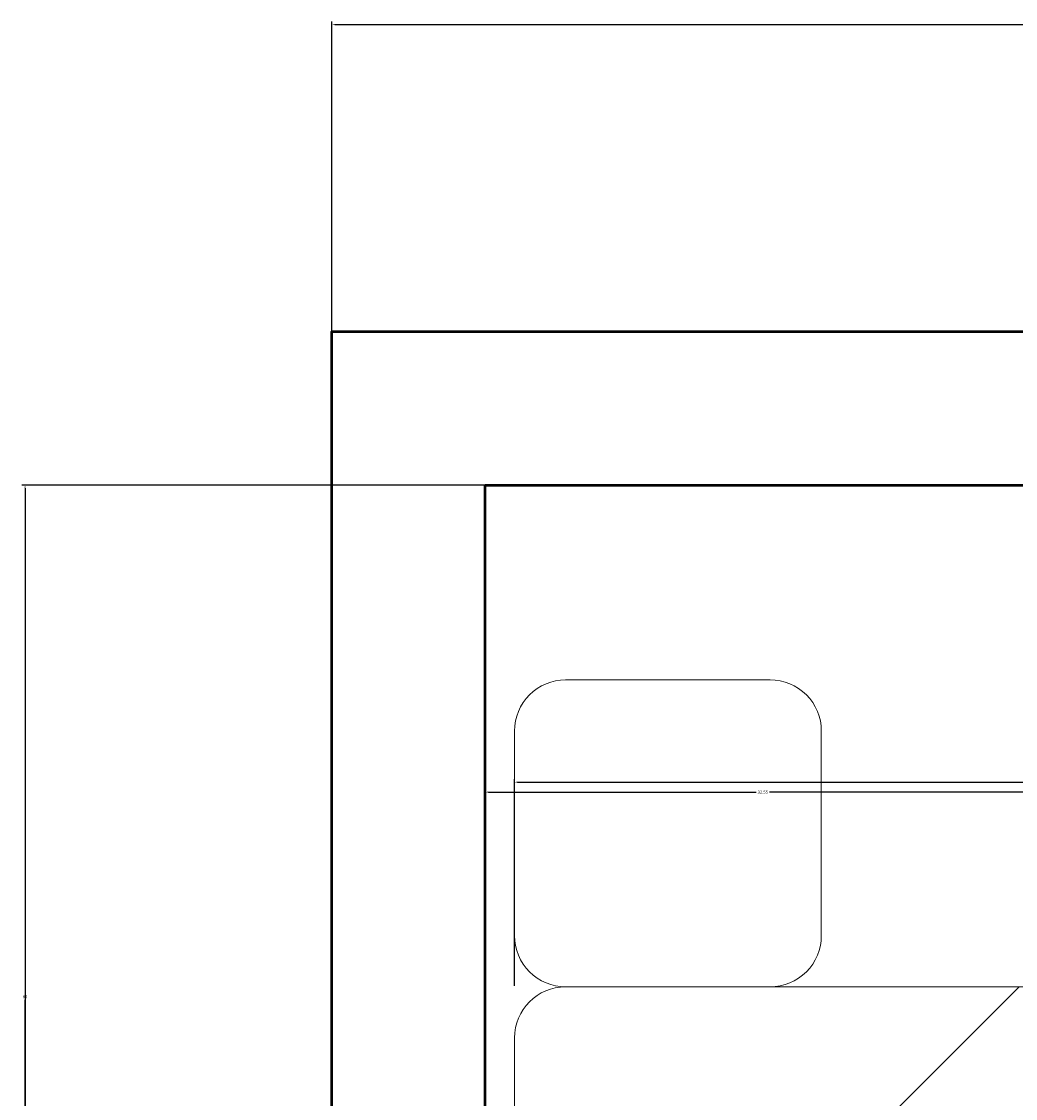
# Model space of a CAD drawing. Units: inches. Extents: x 2621 to 2849, y 2066 to 2463.
# Tile 15 of 28: x 2621 to 2679, y 2399 to 2463. Entities that reach past the tile are written whole.
import ezdxf

# ---------------------------------------------------------------- set-up
doc = ezdxf.new("R2010")
doc.units = ezdxf.units.IN
for name, color, linetype, lineweight in [('A-ANNO-DIMS', 2, 'Continuous', 18), ('A-FURN', 8, 'Continuous', 18), ('A-WALL', 7, 'Continuous', 50)]:
    doc.layers.add(name, color=color, linetype=linetype, lineweight=lineweight)
doc.styles.get("Standard").update_dxf_attribs({"font": 'arial.ttf'})
doc.dimstyles.get("Standard").update_dxf_attribs({"dimtxt": 0.18, "dimasz": 0.18, "dimexe": 0.18, "dimexo": 0.0625, "dimgap": 0.09, "dimtad": 0, "dimtih": 1, "dimtoh": 1, "dimdec": 4, "dimzin": 0, "dimdsep": 46, "dimtxsty": 'Standard', "dimcen": 0.09, "dimadec": 0, "dimazin": 0, "dimtfac": 1, "dimtdec": 4, "dimtofl": 0, "dimtmove": 0, "dimatfit": 3, "dimfxl": 1, "dimtolj": 1, "dimtzin": 0, "dimarcsym": 0})

# ---------------------------------------------------------------- blocks, each defined once
blk = doc.blocks.new('Bed - Queen')
for p, q in [((3, 0), (56.99999, 0)), ((59.99999, -3), (59.99999, -77.00003)), ((59.99999, -29.6), (44.8, -14.4))]:
    blk.add_line(p, q)
blk.add_arc((56.99999, -3), 3, 0, 90)
blk = doc.blocks.new('*D15')
at = {"layer": 'A-ANNO-DIMS', "color": 0, "lineweight": -2, "transparency": 16777216}
for p, q in [((2649.581, 2406.016), (2649.581, 2418.134)), ((2729.581, 2406.016), (2729.581, 2418.134)), ((2649.761, 2417.954), (2688.587, 2417.954)), ((2729.401, 2417.954), (2690.575, 2417.954))]:
    blk.add_line(p, q, dxfattribs=at)
at = {"layer": 'A-ANNO-DIMS', "color": 0, "transparency": 16777216}
for points in [[(2649.761, 2417.984), (2649.761, 2417.924), (2649.581, 2417.954)], [(2729.401, 2417.984), (2729.401, 2417.924), (2729.581, 2417.954)]]:
    blk.add_solid(points, dxfattribs=at)
at = {"layer": 'Defpoints', "color": 0, "transparency": 16777216}
for p in [(2649.581, 2417.954), (2649.581, 2405.954), (2729.581, 2405.954)]:
    blk.add_point(p, dxfattribs=at)
at = {"layer": 'A-ANNO-DIMS', "color": 0, "transparency": 16777216, "insert": (2689.581, 2417.954), "char_height": 0.18, "attachment_point": 5}
blk.add_mtext('\\A1;QUEEN BED 80', dxfattribs=at)
blk = doc.blocks.new('*D35')
at = {"layer": 'A-ANNO-DIMS', "color": 0, "lineweight": -2, "transparency": 16777216}
for p, q in [((2638.87, 2444.437), (2638.87, 2462.558)), ((2639.05, 2462.378), (2734.591, 2462.378)), ((2830.69, 2462.378), (2735.15, 2462.378)), ((2830.87, 2444.437), (2830.87, 2462.558))]:
    blk.add_line(p, q, dxfattribs=at)
at = {"layer": 'A-ANNO-DIMS', "color": 0, "transparency": 16777216}
for points in [[(2639.05, 2462.408), (2639.05, 2462.348), (2638.87, 2462.378)], [(2830.69, 2462.408), (2830.69, 2462.348), (2830.87, 2462.378)]]:
    blk.add_solid(points, dxfattribs=at)
at = {"layer": 'Defpoints', "color": 0, "transparency": 16777216}
for p in [(2830.87, 2462.378), (2638.87, 2444.375), (2830.87, 2444.375)]:
    blk.add_point(p, dxfattribs=at)
at = {"layer": 'A-ANNO-DIMS', "color": 0, "transparency": 16777216, "insert": (2734.87, 2462.378), "char_height": 0.18, "attachment_point": 5}
blk.add_mtext('\\A1;192', dxfattribs=at)
blk = doc.blocks.new('*D37')
at = {"layer": 'A-ANNO-DIMS', "color": 0, "lineweight": -2, "transparency": 16777216}
for p, q in [((2647.87, 2435.312), (2647.87, 2417.191)), ((2680.422, 2435.312), (2680.422, 2417.191)), ((2648.05, 2417.371), (2663.752, 2417.371)), ((2680.242, 2417.371), (2664.54, 2417.371))]:
    blk.add_line(p, q, dxfattribs=at)
at = {"layer": 'A-ANNO-DIMS', "color": 0, "transparency": 16777216}
for points in [[(2648.05, 2417.401), (2648.05, 2417.341), (2647.87, 2417.371)], [(2680.242, 2417.401), (2680.242, 2417.341), (2680.422, 2417.371)]]:
    blk.add_solid(points, dxfattribs=at)
at = {"layer": 'Defpoints', "color": 0, "transparency": 16777216}
for p in [(2647.87, 2435.375), (2680.422, 2435.375), (2647.87, 2417.371)]:
    blk.add_point(p, dxfattribs=at)
at = {"layer": 'A-ANNO-DIMS', "color": 0, "transparency": 16777216, "insert": (2664.146, 2417.371), "char_height": 0.18, "attachment_point": 5}
blk.add_mtext('\\A1;32.55', dxfattribs=at)
blk = doc.blocks.new('*D46')
at = {"layer": 'A-ANNO-DIMS', "color": 0, "lineweight": -2, "transparency": 16777216}
for p, q in [((2647.808, 2435.375), (2620.687, 2435.375)), ((2620.867, 2435.195), (2620.867, 2377.556)), ((2620.867, 2319.555), (2620.867, 2377.193)), ((2647.808, 2319.375), (2620.687, 2319.375))]:
    blk.add_line(p, q, dxfattribs=at)
at = {"layer": 'A-ANNO-DIMS', "color": 0, "transparency": 16777216}
for points in [[(2620.837, 2435.195), (2620.897, 2435.195), (2620.867, 2435.375)], [(2620.837, 2319.555), (2620.897, 2319.555), (2620.867, 2319.375)]]:
    blk.add_solid(points, dxfattribs=at)
at = {"layer": 'Defpoints', "color": 0, "transparency": 16777216}
for p in [(2620.867, 2435.375), (2647.87, 2435.375), (2647.87, 2319.375)]:
    blk.add_point(p, dxfattribs=at)
at = {"layer": 'A-ANNO-DIMS', "color": 0, "transparency": 16777216, "insert": (2620.867, 2377.375), "char_height": 0.18, "attachment_point": 5}
blk.add_mtext('\\A1;116', dxfattribs=at)
blk = doc.blocks.new('*D68')
at = {"layer": 'A-ANNO-DIMS', "color": 0, "lineweight": -2, "transparency": 16777216}
for p, q in [((2745.808, 2435.375), (2620.687, 2435.375)), ((2620.867, 2435.195), (2620.867, 2405.556)), ((2620.867, 2375.555), (2620.867, 2405.193)), ((2745.808, 2375.375), (2620.687, 2375.375))]:
    blk.add_line(p, q, dxfattribs=at)
at = {"layer": 'A-ANNO-DIMS', "color": 0, "transparency": 16777216}
for points in [[(2620.837, 2435.195), (2620.897, 2435.195), (2620.867, 2435.375)], [(2620.837, 2375.555), (2620.897, 2375.555), (2620.867, 2375.375)]]:
    blk.add_solid(points, dxfattribs=at)
at = {"layer": 'Defpoints', "color": 0, "transparency": 16777216}
for p in [(2620.867, 2435.375), (2745.87, 2435.375), (2745.87, 2375.375)]:
    blk.add_point(p, dxfattribs=at)
at = {"layer": 'A-ANNO-DIMS', "color": 0, "transparency": 16777216, "insert": (2620.867, 2405.375), "char_height": 0.18, "attachment_point": 5}
blk.add_mtext('\\A1;60', dxfattribs=at)

msp = doc.modelspace()

# ---------------------------------------------------------------- linework, layer by layer
at = {"layer": 'A-FURN'}
msp.add_lwpolyline([(2652.5811, 2405.9537), (2664.5811, 2405.9537, 0.4142136), (2667.5811, 2408.9537), (2667.5811, 2420.9537, 0.4142136), (2664.5811, 2423.9537), (2652.5811, 2423.9537, 0.4142136), (2649.5811, 2420.9537), (2649.5811, 2408.9537, 0.4142136)], format="xyb", close=True, dxfattribs=at)
at = {"layer": 'A-WALL'}
for p, q in [((2647.8701, 2435.3746), (2763.8701, 2435.3746)), ((2647.8701, 2319.3746), (2647.8701, 2435.3746))]:
    msp.add_line(p, q, dxfattribs=at)
msp.add_lwpolyline([(2761.8701, 2084.3746), (2638.8701, 2084.3746), (2638.8701, 2444.3746), (2830.8701, 2444.3746), (2830.8701, 2084.3746), (2797.8701, 2084.3746)], dxfattribs=at)

# ---------------------------------------------------------------- block references
at = {"layer": 'A-FURN', "rotation": 90}
msp.add_blockref('Bed - Queen', (2649.5811, 2345.9537), dxfattribs=at)

# ---------------------------------------------------------------- dimensions: what is measured, and where the dimension line sits
at = {"layer": 'A-ANNO-DIMS'}
dim = msp.add_linear_dim(base=(2830.8701, 2462.3781), p1=(2638.8701, 2444.3746), p2=(2830.8701, 2444.3746), dimstyle='Standard', override={"dimdec": 0, "dimlfac": 1, "dimrnd": 0, "dimzin": 0, "dimdsep": 46, "dimlunit": 2}, dxfattribs=at)
dim.commit()
dim.dimension.update_dxf_attribs({"geometry": '*D35', "text_midpoint": (2734.8701, 2462.3781)})
for base, p1, p2, angle, override, picture, middle in [((2620.8666, 2435.3746), (2647.8701, 2319.3746), (2647.8701, 2435.3746), 90, {"dimdec": 0, "dimlfac": 1, "dimrnd": 0, "dimzin": 0, "dimdsep": 46, "dimlunit": 2}, '*D46', (2620.8666, 2377.3746)), ((2620.8666, 2435.3746), (2745.8701, 2375.3746), (2745.8701, 2435.3746), 90, {"dimdec": 0, "dimlfac": 1, "dimrnd": 0, "dimzin": 0, "dimdsep": 46, "dimlunit": 2}, '*D68', (2620.8666, 2405.3746)), ((2647.8701, 2417.3711), (2680.4219, 2435.3746), (2647.8701, 2435.3746), 180, {"dimdec": 2, "dimlfac": 1, "dimrnd": 0, "dimzin": 0, "dimdsep": 46, "dimlunit": 2}, '*D37', (2664.146, 2417.3711))]:
    dim = msp.add_linear_dim(base=base, p1=p1, p2=p2, angle=angle, dimstyle='Standard', override=override, dxfattribs=at)
    dim.commit()
    dim.dimension.update_dxf_attribs({"geometry": picture, "text_midpoint": middle})
dim = msp.add_linear_dim(base=(2649.5811, 2417.9537), p1=(2729.5811, 2405.9537), p2=(2649.5811, 2405.9537), angle=180, text='QUEEN BED <>', dimstyle='Standard', override={"dimdec": 0, "dimlfac": 1, "dimrnd": 0, "dimzin": 0, "dimdsep": 46, "dimlunit": 2}, dxfattribs=at)
dim.commit()
dim.dimension.update_dxf_attribs({"geometry": '*D15', "text_midpoint": (2689.5811, 2417.9537)})

doc.saveas('drawing.dxf')
